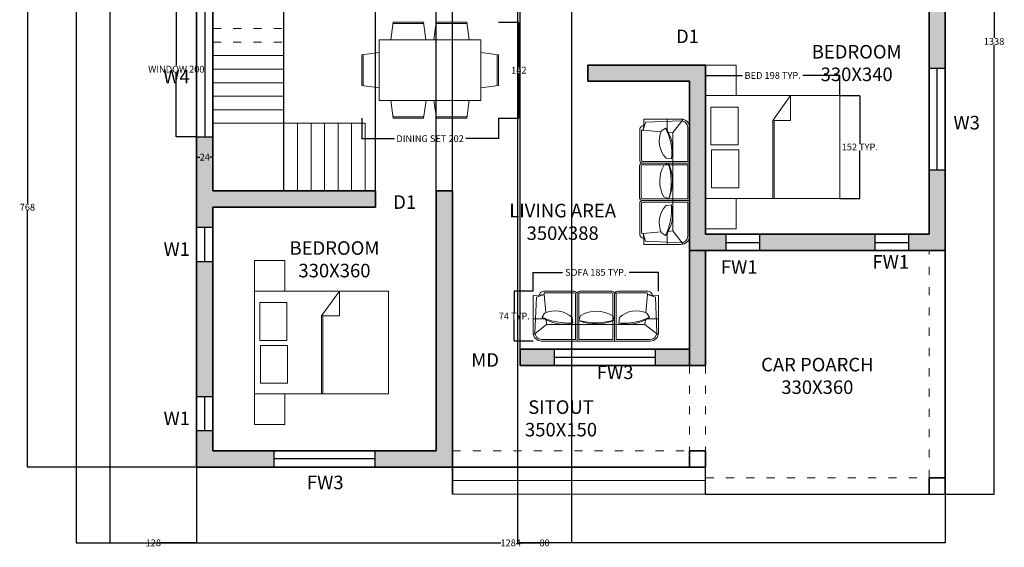
# Model space of a CAD drawing. Units: centimetres. Extents: x 1399 to 2860, y -110 to 1386.
# Tile 1 of 3: x 1399 to 2854, y -110 to 670. Entities that reach past the tile are written whole.
import ezdxf

# ---------------------------------------------------------------- set-up
doc = ezdxf.new("R2010")
doc.units = ezdxf.units.CM
doc.header["$MEASUREMENT"] = 0
doc.linetypes.add('ACAD_ISO03W100', pattern=[30, 12, -18])
for name, color, linetype, lineweight in [('A-ANNO-DIMS', 2, 'Continuous', 18), ('A-ANNO-TEXT', 7, 'Continuous', 18), ('A-AREA-IDEN', 7, 'Continuous', 25), ('A-COLS', 7, 'Continuous', 35), ('A-FLOR', 7, 'Continuous', 25), ('A-FLOR-OVHD', 8, 'ACAD_ISO03W100', 18), ('A-FLOR-STRS', 7, 'Continuous', 18), ('A-FLOR-STRS-OVHD', 8, 'ACAD_ISO03W100', 18), ('A-FURN', 8, 'Continuous', 18), ('A-GLAZ', 4, 'Continuous', 25), ('A-WALL', 7, 'Continuous', 35), ('A-WALL-PATT', 252, 'Continuous', 13)]:
    doc.layers.add(name, color=color, linetype=linetype, lineweight=lineweight)
doc.styles.get("Standard").update_dxf_attribs({"font": 'arial.ttf'})
doc.dimstyles.get("Standard").update_dxf_attribs({"dimtxt": 10, "dimasz": 0.18, "dimexe": 0.18, "dimexo": 0.0625, "dimgap": 0.09, "dimtad": 0, "dimtih": 1, "dimtoh": 1, "dimdec": 4, "dimzin": 0, "dimdsep": 46, "dimtxsty": 'Standard', "dimcen": 0.09, "dimadec": 0, "dimazin": 0, "dimtfac": 1, "dimtdec": 4, "dimtofl": 0, "dimtmove": 0, "dimatfit": 3, "dimfxl": 1, "dimtolj": 1, "dimtzin": 0, "dimarcsym": 0})

# ---------------------------------------------------------------- blocks, each defined once
blk = doc.blocks.new('v')
blk.add_line((1187.1, 1404.2), (1237.1, 1404.2))
blk.add_lwpolyline([(1187.1, 1392.2), (1237.1, 1392.2), (1237.1, 1416.2), (1187.1, 1416.2)], close=True)
blk = doc.blocks.new('w3')
blk.add_line((1235.3, 1319.4), (1085.3, 1319.4))
blk.add_lwpolyline([(1085.3, 1307.4), (1235.3, 1307.4), (1235.3, 1331.4), (1085.3, 1331.4)], close=True)
blk = doc.blocks.new('A$C7EC0217F')
for p, q in [((0.135, 0.808), (0.711, 0.808)), ((0.711, 0.808), (0.711, 0.046)), ((0.711, 0.807), (1.319, 0.807)), ((0.711, 0.045), (0.711, 0.807)), ((1.319, 0.807), (1.319, 0.045)), ((1.32, 0.808), (1.32, 0.046)), ((1.896, 0.808), (1.32, 0.808)), ((0, 0.069), (0, 0.673)), ((0.218, 0.538), (0.004, 0.706)), ((0.027, 0.673), (0.047, 0.095)), ((0.135, 0.781), (0.684, 0.781)), ((0.684, 0.045), (0.684, 0.781)), ((0.738, 0.78), (1.292, 0.78)), ((0.738, 0.045), (0.738, 0.78)), ((1.292, 0.78), (1.292, 0.045)), ((1.346, 0.781), (1.346, 0.045)), ((1.896, 0.781), (1.346, 0.781)), ((1.813, 0.538), (2.027, 0.706)), ((2.004, 0.673), (1.977, 0.095)), ((2.031, 0.069), (2.031, 0.673)), ((0.212, 0.464), (0.218, 0.538)), ((0.218, 0.538), (0.711, 0.538)), ((0.632, 0.428), (0.644, 0.516)), ((0.711, 0.612), (0.711, 0.612)), ((0.711, 0.537), (1.319, 0.537)), ((1.32, 0.612), (1.319, 0.612)), ((1.813, 0.538), (1.32, 0.538)), ((1.399, 0.428), (1.388, 0.516)), ((1.819, 0.464), (1.813, 0.538)), ((0, 0.448), (0.185, 0.448)), ((0.144, 0.42), (0.187, 0.355)), ((0.18, 0.055), (0.203, 0.347)), ((0.711, 0.432), (0.711, 0.432)), ((0.712, 0.47), (0.742, 0.399)), ((1.261, 0.391), (1.288, 0.475)), ((1.32, 0.432), (1.319, 0.432)), ((1.852, 0.055), (1.828, 0.347)), ((1.887, 0.42), (1.845, 0.355)), ((2.031, 0.448), (1.847, 0.448)), ((0.1, 0.066), (0, 0.069)), ((0.047, 0.095), (0.18, 0.055)), ((0.1, 0.066), (0.18, 0.055)), ((0.181, 0.028), (0.18, 0.055)), ((0.666, 0.028), (0.181, 0.028)), ((0.666, 0.001), (0.181, 0.001)), ((1.274, 0.027), (0.756, 0.027)), ((1.274, 0), (0.756, 0)), ((1.365, 0.028), (1.85, 0.028)), ((1.365, 0.001), (1.85, 0.001)), ((1.85, 0.028), (1.852, 0.055)), ((1.977, 0.095), (1.852, 0.055)), ((1.932, 0.066), (1.852, 0.055)), ((1.932, 0.066), (2.031, 0.069))]:
    blk.add_line(p, q)
for centre, radius, start, end in [((0.135, 0.673), 0.135, 90, 180), ((1.896, 0.673), 0.135, 0, 90), ((0.135, 0.673), 0.108, 90, 180), ((1.896, 0.673), 0.108, 0, 90), ((0.493, -0.046), 0.581, 74.928, 126.7929), ((0.559, -0.39), 0.91, 84.6406, 117.0804), ((1.02, -0.477), 0.989, 74.3176, 108.1894), ((1.006, -0.207), 0.738, 67.5209, 113.4724), ((1.381, -1.331), 1.892, 91.8503, 91.8916), ((1.381, -1.331), 1.87, 91.8726, 91.9144), ((1.539, -0.046), 0.581, 53.2071, 105.072), ((1.446, -0.529), 1.046, 65.0725, 93.2065), ((0.356, 0.715), 0.398, 244.7866, 313.8058), ((1.314, -1.331), 1.892, 108.5655, 108.5801), ((1.314, -1.331), 1.87, 108.7972, 108.812), ((1.008, 0.84), 0.515, 238.8934, 299.3642), ((1.675, 0.715), 0.398, 226.1942, 295.2134), ((1.381, -1.391), 1.6, 92.1888, 92.2376), ((0.173, 0.074), 0.0734, 186.4251, 276.5821), ((0.666, 0.046), 0.045, 270, 0), ((0.666, 0.046), 0.018, 270, 0), ((0.756, 0.045), 0.045, 180, 270), ((0.756, 0.045), 0.018, 180, 270), ((1.274, 0.045), 0.045, 270, 0), ((1.274, 0.045), 0.018, 270, 0), ((1.381, -1.391), 1.51, 92.3193, 92.3711), ((1.365, 0.046), 0.045, 180, 270), ((1.365, 0.046), 0.018, 180, 270), ((1.859, 0.074), 0.0734, 263.4179, 353.5749)]:
    blk.add_arc(centre, radius, start, end)
blk = doc.blocks.new('BED')
for p, q in [((1734.1, 2886.7), (1849.5, 2886.7)), ((1734.1, 2884.7), (1849.5, 2884.7)), ((1849.5, 2886.7), (1886.1, 2860.2)), ((1886.1, 2860.2), (1849.5, 2886.7)), ((1849.5, 2886.7), (1849.5, 2860.2)), ((1849.5, 2860.2), (1886.1, 2860.2))]:
    blk.add_line(p, q)
for points in [[(1734.1, 2787.7), (1886.1, 2787.7), (1886.1, 2985.7), (1734.1, 2985.7)], [(1750, 2936.8), (1805.9, 2936.8), (1805.9, 2977), (1750, 2977)], [(1813.2, 2937.8), (1869.1, 2937.8), (1869.1, 2977.9), (1813.2, 2977.9)]]:
    blk.add_lwpolyline(points, close=True)
blk = doc.blocks.new('DINING')
for p, q in [((1379.7, 3775.6), (1376.2, 3749.7)), ((1379.7, 3775.6), (1424.7, 3775.6)), ((1379.7, 3773.6), (1424.7, 3773.6)), ((1424.7, 3775.6), (1428.2, 3749.7)), ((1443.5, 3775.6), (1440, 3749.7)), ((1443.5, 3775.6), (1488.5, 3775.6)), ((1443.5, 3773.6), (1488.5, 3773.6)), ((1488.5, 3775.6), (1492, 3749.7)), ((1376.2, 3749.7), (1428.2, 3749.7)), ((1440, 3749.7), (1492, 3749.7)), ((1333.4, 3727.2), (1359.3, 3730.7)), ((1333.4, 3682.2), (1333.4, 3727.2)), ((1335.4, 3682.2), (1335.4, 3727.2)), ((1359.3, 3678.7), (1359.3, 3730.7)), ((1509.3, 3730.7), (1509.3, 3678.7)), ((1535.2, 3727.2), (1509.3, 3730.7)), ((1533.2, 3727.2), (1533.2, 3682.2)), ((1535.2, 3727.2), (1535.2, 3682.2)), ((1333.4, 3682.2), (1359.3, 3678.7)), ((1535.2, 3682.2), (1509.3, 3678.7)), ((1428.3, 3659.7), (1376.3, 3659.7)), ((1379.8, 3633.8), (1376.3, 3659.7)), ((1424.8, 3633.8), (1428.3, 3659.7)), ((1492.1, 3659.7), (1440.1, 3659.7)), ((1443.6, 3633.8), (1440.1, 3659.7)), ((1488.6, 3633.8), (1492.1, 3659.7)), ((1424.8, 3635.8), (1379.8, 3635.8)), ((1424.8, 3633.8), (1379.8, 3633.8)), ((1488.6, 3635.8), (1443.6, 3635.8)), ((1488.6, 3633.8), (1443.6, 3633.8))]:
    blk.add_line(p, q)
blk.add_lwpolyline([(1359.3, 3659.7), (1509.3, 3659.7), (1509.3, 3749.7), (1359.3, 3749.7)], close=True)
blk = doc.blocks.new('W4')
blk.add_line((1292.5, 2297.5), (1492.5, 2297.5))
blk.add_lwpolyline([(1292.5, 2285.5), (1492.5, 2285.5), (1492.5, 2309.5), (1292.5, 2309.5)], close=True)
blk = doc.blocks.new('NIGHTSTAND-450')
blk.add_lwpolyline([(0, 45), (0, 0), (45, 0), (45, 45)], close=True)
blk = doc.blocks.new('*D21')
at = {"layer": 'A-ANNO-DIMS', "color": 0, "lineweight": -2, "transparency": 16777216}
for p, q in [((1660.7, 697), (1630.6, 697)), ((1630.8, 696.8), (1630.8, 602.3)), ((1630.8, 497.2), (1630.8, 591.7)), ((1660.7, 497), (1630.6, 497))]:
    blk.add_line(p, q, dxfattribs=at)
at = {"layer": 'A-ANNO-DIMS', "color": 0, "transparency": 16777216}
for points in [[(1630.8, 696.8), (1630.8, 696.8), (1630.8, 697)], [(1630.8, 497.2), (1630.8, 497.2), (1630.8, 497)]]:
    blk.add_solid(points, dxfattribs=at)
at = {"layer": 'Defpoints', "color": 0, "transparency": 16777216}
for p in [(1660.8, 697), (1630.8, 497), (1660.8, 497)]:
    blk.add_point(p, dxfattribs=at)
at = {"layer": 'A-ANNO-DIMS', "color": 0, "transparency": 16777216, "insert": (1630.8, 597), "char_height": 10, "attachment_point": 5}
blk.add_mtext('\\A1;WINDOW 200', dxfattribs=at)
blk = doc.blocks.new('*D22')
at = {"layer": 'A-ANNO-DIMS', "color": 0, "lineweight": -2, "transparency": 16777216}
for p, q in [((1660.8, 496.9), (1660.8, 466.8)), ((1684.8, 496.9), (1684.8, 466.8)), ((1661, 467), (1665.5, 467)), ((1684.6, 467), (1680.1, 467))]:
    blk.add_line(p, q, dxfattribs=at)
at = {"layer": 'A-ANNO-DIMS', "color": 0, "transparency": 16777216}
for points in [[(1661, 467), (1661, 467), (1660.8, 467)], [(1684.6, 467), (1684.6, 467), (1684.8, 467)]]:
    blk.add_solid(points, dxfattribs=at)
at = {"layer": 'Defpoints', "color": 0, "transparency": 16777216}
for p in [(1660.8, 497), (1684.8, 497), (1684.8, 467)]:
    blk.add_point(p, dxfattribs=at)
at = {"layer": 'A-ANNO-DIMS', "color": 0, "transparency": 16777216, "insert": (1672.8, 467), "char_height": 10, "attachment_point": 5}
blk.add_mtext('\\A1;24', dxfattribs=at)
blk = doc.blocks.new('*D23')
at = {"layer": 'A-ANNO-DIMS', "color": 0, "lineweight": -2, "transparency": 16777216}
for p, q in [((2412.8, 558.1), (2412.8, 587.9)), ((2413, 587.7), (2467.4, 587.7)), ((2610.6, 587.7), (2556.2, 587.7)), ((2610.8, 558.1), (2610.8, 587.9))]:
    blk.add_line(p, q, dxfattribs=at)
at = {"layer": 'A-ANNO-DIMS', "color": 0, "transparency": 16777216}
for points in [[(2413, 587.7), (2413, 587.7), (2412.8, 587.7)], [(2610.6, 587.7), (2610.6, 587.7), (2610.8, 587.7)]]:
    blk.add_solid(points, dxfattribs=at)
at = {"layer": 'Defpoints', "color": 0, "transparency": 16777216}
for p in [(2412.8, 587.7), (2412.8, 558), (2610.8, 558)]:
    blk.add_point(p, dxfattribs=at)
at = {"layer": 'A-ANNO-DIMS', "color": 0, "transparency": 16777216, "insert": (2511.8, 587.7), "char_height": 10, "attachment_point": 5}
blk.add_mtext('\\A1;BED 198 TYP.', dxfattribs=at)
blk = doc.blocks.new('*D24')
at = {"layer": 'A-ANNO-DIMS', "color": 0, "lineweight": -2, "transparency": 16777216}
for p, q in [((2610.9, 558), (2640.7, 558)), ((2640.5, 557.8), (2640.5, 487.2)), ((2640.5, 406.2), (2640.5, 476.8)), ((2610.9, 406), (2640.7, 406))]:
    blk.add_line(p, q, dxfattribs=at)
at = {"layer": 'A-ANNO-DIMS', "color": 0, "transparency": 16777216}
for points in [[(2640.5, 557.8), (2640.5, 557.8), (2640.5, 558)], [(2640.5, 406.2), (2640.5, 406.2), (2640.5, 406)]]:
    blk.add_solid(points, dxfattribs=at)
at = {"layer": 'Defpoints', "color": 0, "transparency": 16777216}
for p in [(2610.8, 558), (2640.5, 558), (2610.8, 406)]:
    blk.add_point(p, dxfattribs=at)
at = {"layer": 'A-ANNO-DIMS', "color": 0, "transparency": 16777216, "insert": (2640.5, 482), "char_height": 10, "attachment_point": 5}
blk.add_mtext('\\A1;152 TYP.', dxfattribs=at)
blk = doc.blocks.new('*D29')
at = {"layer": 'A-ANNO-DIMS', "color": 0, "lineweight": -2, "transparency": 16777216}
for p, q in [((2157.9, 269), (2157.9, 296.9)), ((2158.1, 296.7), (2201.2, 296.7)), ((2342.9, 296.7), (2299.7, 296.7)), ((2343, 269), (2343, 296.9))]:
    blk.add_line(p, q, dxfattribs=at)
at = {"layer": 'A-ANNO-DIMS', "color": 0, "transparency": 16777216}
for points in [[(2158.1, 296.7), (2158.1, 296.7), (2157.9, 296.7)], [(2342.9, 296.7), (2342.9, 296.7), (2343, 296.7)]]:
    blk.add_solid(points, dxfattribs=at)
at = {"layer": 'Defpoints', "color": 0, "transparency": 16777216}
for p in [(2157.9, 296.7), (2157.9, 268.9), (2343, 268.9)]:
    blk.add_point(p, dxfattribs=at)
at = {"layer": 'A-ANNO-DIMS', "color": 0, "transparency": 16777216, "insert": (2250.5, 296.7), "char_height": 10, "attachment_point": 5}
blk.add_mtext('\\A1;SOFA 185 TYP.', dxfattribs=at)
blk = doc.blocks.new('*D30')
at = {"layer": 'A-ANNO-DIMS', "color": 0, "lineweight": -2, "transparency": 16777216}
for p, q in [((2157.8, 268.9), (2130, 268.9)), ((2130.1, 268.8), (2130.1, 237.2)), ((2130.1, 195.4), (2130.1, 227)), ((2157.8, 195.2), (2130, 195.2))]:
    blk.add_line(p, q, dxfattribs=at)
at = {"layer": 'A-ANNO-DIMS', "color": 0, "transparency": 16777216}
for points in [[(2130.1, 268.8), (2130.2, 268.8), (2130.1, 268.9)], [(2130.1, 195.4), (2130.2, 195.4), (2130.1, 195.2)]]:
    blk.add_solid(points, dxfattribs=at)
at = {"layer": 'Defpoints', "color": 0, "transparency": 16777216}
for p in [(2157.9, 268.9), (2130.1, 195.2), (2157.9, 195.2)]:
    blk.add_point(p, dxfattribs=at)
at = {"layer": 'A-ANNO-DIMS', "color": 0, "transparency": 16777216, "insert": (2130.1, 232.1), "char_height": 10, "attachment_point": 5}
blk.add_mtext('\\A1;74 TYP.', dxfattribs=at)
blk = doc.blocks.new('*D31')
at = {"layer": 'A-ANNO-DIMS', "color": 0, "lineweight": -2, "transparency": 16777216}
for p, q in [((1904.8, 524.5), (1904.8, 494.1)), ((2106.6, 524.5), (2106.6, 494.1)), ((1905, 494.3), (1952.9, 494.3)), ((2106.4, 494.3), (2058.4, 494.3))]:
    blk.add_line(p, q, dxfattribs=at)
at = {"layer": 'A-ANNO-DIMS', "color": 0, "transparency": 16777216}
for points in [[(1905, 494.3), (1905, 494.3), (1904.8, 494.3)], [(2106.4, 494.3), (2106.4, 494.3), (2106.6, 494.3)]]:
    blk.add_solid(points, dxfattribs=at)
at = {"layer": 'Defpoints', "color": 0, "transparency": 16777216}
for p in [(1904.8, 524.6), (2106.6, 524.6), (2106.6, 494.3)]:
    blk.add_point(p, dxfattribs=at)
at = {"layer": 'A-ANNO-DIMS', "color": 0, "transparency": 16777216, "insert": (2005.7, 494.3), "char_height": 10, "attachment_point": 5}
blk.add_mtext('\\A1;DINING SET 202', dxfattribs=at)
blk = doc.blocks.new('*D32')
at = {"layer": 'A-ANNO-DIMS', "color": 0, "lineweight": -2, "transparency": 16777216}
for p, q in [((2106.6, 666.4), (2137, 666.4)), ((2136.8, 666.2), (2136.8, 600.6)), ((2136.8, 524.8), (2136.8, 590.4)), ((2106.6, 524.6), (2137, 524.6))]:
    blk.add_line(p, q, dxfattribs=at)
at = {"layer": 'A-ANNO-DIMS', "color": 0, "transparency": 16777216}
for points in [[(2136.8, 666.2), (2136.9, 666.2), (2136.8, 666.4)], [(2136.8, 524.8), (2136.9, 524.8), (2136.8, 524.6)]]:
    blk.add_solid(points, dxfattribs=at)
at = {"layer": 'Defpoints', "color": 0, "transparency": 16777216}
for p in [(2106.6, 666.4), (2136.8, 666.4), (2106.6, 524.6)]:
    blk.add_point(p, dxfattribs=at)
at = {"layer": 'A-ANNO-DIMS', "color": 0, "transparency": 16777216, "insert": (2136.8, 595.5), "char_height": 10, "attachment_point": 5}
blk.add_mtext('\\A1;142', dxfattribs=at)
blk = doc.blocks.new('*D37')
at = {"layer": 'A-ANNO-DIMS', "color": 0, "lineweight": -2, "transparency": 16777216}
for p, q in [((1482.8, 800.9), (1482.8, -103.2)), ((2766.8, -31.1), (2766.8, -103.2)), ((1483, -103), (2110.3, -103)), ((2766.6, -103), (2139.3, -103))]:
    blk.add_line(p, q, dxfattribs=at)
at = {"layer": 'A-ANNO-DIMS', "color": 0, "transparency": 16777216}
for points in [[(1483, -103), (1483, -103.1), (1482.8, -103)], [(2766.6, -103), (2766.6, -103.1), (2766.8, -103)]]:
    blk.add_solid(points, dxfattribs=at)
at = {"layer": 'Defpoints', "color": 0, "transparency": 16777216}
for p in [(1482.8, 801), (2766.8, -31), (2766.8, -103)]:
    blk.add_point(p, dxfattribs=at)
at = {"layer": 'A-ANNO-DIMS', "color": 0, "transparency": 16777216, "insert": (2124.8, -103), "char_height": 10, "attachment_point": 5}
blk.add_mtext('\\A1;1284', dxfattribs=at)
blk = doc.blocks.new('*D38')
at = {"layer": 'A-ANNO-DIMS', "color": 0, "lineweight": -2, "transparency": 16777216}
for p, q in [((2766.9, 1307), (2839, 1307)), ((2838.9, 1306.8), (2838.9, 643.2)), ((2838.9, -30.8), (2838.9, 632.8)), ((2766.9, -31), (2839, -31))]:
    blk.add_line(p, q, dxfattribs=at)
at = {"layer": 'A-ANNO-DIMS', "color": 0, "transparency": 16777216}
for points in [[(2838.8, 1306.8), (2838.9, 1306.8), (2838.9, 1307)], [(2838.8, -30.8), (2838.9, -30.8), (2838.9, -31)]]:
    blk.add_solid(points, dxfattribs=at)
at = {"layer": 'Defpoints', "color": 0, "transparency": 16777216}
for p in [(2766.8, 1307), (2838.9, 1307), (2766.8, -31)]:
    blk.add_point(p, dxfattribs=at)
at = {"layer": 'A-ANNO-DIMS', "color": 0, "transparency": 16777216, "insert": (2838.9, 638), "char_height": 10, "attachment_point": 5}
blk.add_mtext('\\A1;1338', dxfattribs=at)
blk = doc.blocks.new('*D41')
at = {"layer": 'A-ANNO-DIMS', "color": 0, "lineweight": -2, "transparency": 16777216}
for p, q in [((1532.8, 776.9), (1532.8, -103.2)), ((1660.8, 776.9), (1660.8, -103.2)), ((1533, -103), (1586.1, -103)), ((1660.6, -103), (1607.5, -103))]:
    blk.add_line(p, q, dxfattribs=at)
at = {"layer": 'A-ANNO-DIMS', "color": 0, "transparency": 16777216}
for points in [[(1533, -103), (1533, -103.1), (1532.8, -103)], [(1660.6, -103), (1660.6, -103.1), (1660.8, -103)]]:
    blk.add_solid(points, dxfattribs=at)
at = {"layer": 'Defpoints', "color": 0, "transparency": 16777216}
for p in [(1532.8, 777), (1660.8, 777), (1660.8, -103)]:
    blk.add_point(p, dxfattribs=at)
at = {"layer": 'A-ANNO-DIMS', "color": 0, "transparency": 16777216, "insert": (1596.8, -103), "char_height": 10, "attachment_point": 5}
blk.add_mtext('\\A1;128', dxfattribs=at)
blk = doc.blocks.new('*D43')
at = {"layer": 'A-ANNO-DIMS', "color": 0, "lineweight": -2, "transparency": 16777216}
for p, q in [((1924.8, 417.1), (1924.8, 1379.2)), ((1925, 1379.1), (1962.6, 1379.1)), ((2014.6, 1379.1), (1977, 1379.1)), ((2014.8, 417.1), (2014.8, 1379.2))]:
    blk.add_line(p, q, dxfattribs=at)
at = {"layer": 'A-ANNO-DIMS', "color": 0, "transparency": 16777216}
for points in [[(1925, 1379.1), (1925, 1379), (1924.8, 1379.1)], [(2014.6, 1379.1), (2014.6, 1379), (2014.8, 1379.1)]]:
    blk.add_solid(points, dxfattribs=at)
at = {"layer": 'Defpoints', "color": 0, "transparency": 16777216}
for p in [(2014.8, 1379.1), (1924.8, 417), (2014.8, 417)]:
    blk.add_point(p, dxfattribs=at)
at = {"layer": 'A-ANNO-DIMS', "color": 0, "transparency": 16777216, "insert": (1969.8, 1379.1), "char_height": 10, "attachment_point": 5}
blk.add_mtext('\\A1;90', dxfattribs=at)
blk = doc.blocks.new('*D44')
at = {"layer": 'A-ANNO-DIMS', "color": 0, "lineweight": -2, "transparency": 16777216}
for p, q in [((2134.8, 906.9), (2134.8, -103.2)), ((2214.8, 906.9), (2214.8, -103.2)), ((2135, -103), (2167.6, -103)), ((2214.6, -103), (2182, -103))]:
    blk.add_line(p, q, dxfattribs=at)
at = {"layer": 'A-ANNO-DIMS', "color": 0, "transparency": 16777216}
for points in [[(2135, -103), (2135, -103.1), (2134.8, -103)], [(2214.6, -103), (2214.6, -103.1), (2214.8, -103)]]:
    blk.add_solid(points, dxfattribs=at)
at = {"layer": 'Defpoints', "color": 0, "transparency": 16777216}
for p in [(2134.8, 907), (2214.8, 907), (2214.8, -103)]:
    blk.add_point(p, dxfattribs=at)
at = {"layer": 'A-ANNO-DIMS', "color": 0, "transparency": 16777216, "insert": (2174.8, -103), "char_height": 10, "attachment_point": 5}
blk.add_mtext('\\A1;80', dxfattribs=at)
blk = doc.blocks.new('*D45')
at = {"layer": 'A-ANNO-DIMS', "color": 0, "lineweight": -2, "transparency": 16777216}
for p, q in [((2038.8, 33.1), (2038.8, 1379.2)), ((2039, 1379.1), (2078.2, 1379.1)), ((2138.6, 1379.1), (2099.5, 1379.1)), ((2138.8, 183.1), (2138.8, 1379.2))]:
    blk.add_line(p, q, dxfattribs=at)
at = {"layer": 'A-ANNO-DIMS', "color": 0, "transparency": 16777216}
for points in [[(2039, 1379.1), (2039, 1379), (2038.8, 1379.1)], [(2138.6, 1379.1), (2138.6, 1379), (2138.8, 1379.1)]]:
    blk.add_solid(points, dxfattribs=at)
at = {"layer": 'Defpoints', "color": 0, "transparency": 16777216}
for p in [(2038.8, 1379.1), (2138.8, 183), (2038.8, 33)]:
    blk.add_point(p, dxfattribs=at)
at = {"layer": 'A-ANNO-DIMS', "color": 0, "transparency": 16777216, "insert": (2088.8, 1379.1), "char_height": 10, "attachment_point": 5}
blk.add_mtext('\\A1;100', dxfattribs=at)
blk = doc.blocks.new('*D48')
at = {"layer": 'A-ANNO-DIMS', "color": 0, "lineweight": -2, "transparency": 16777216}
for p, q in [((1684.8, 417.1), (1684.8, 1379.2)), ((1685, 1379.1), (1726.6, 1379.1)), ((1789.6, 1379.1), (1748, 1379.1)), ((1789.8, 417.1), (1789.8, 1379.2))]:
    blk.add_line(p, q, dxfattribs=at)
at = {"layer": 'A-ANNO-DIMS', "color": 0, "transparency": 16777216}
for points in [[(1685, 1379.1), (1685, 1379), (1684.8, 1379.1)], [(1789.6, 1379.1), (1789.6, 1379), (1789.8, 1379.1)]]:
    blk.add_solid(points, dxfattribs=at)
at = {"layer": 'Defpoints', "color": 0, "transparency": 16777216}
for p in [(1789.8, 1379.1), (1684.8, 417), (1789.8, 417)]:
    blk.add_point(p, dxfattribs=at)
at = {"layer": 'A-ANNO-DIMS', "color": 0, "transparency": 16777216, "insert": (1737.3, 1379.1), "char_height": 10, "attachment_point": 5}
blk.add_mtext('\\A1;105', dxfattribs=at)
blk = doc.blocks.new('*D50')
at = {"layer": 'A-ANNO-DIMS', "color": 0, "lineweight": -2, "transparency": 16777216}
for p, q in [((1660.7, 777), (1410.6, 777)), ((1410.8, 776.8), (1410.8, 398.2)), ((1410.8, 9.2), (1410.8, 387.8)), ((1660.7, 9), (1410.6, 9))]:
    blk.add_line(p, q, dxfattribs=at)
at = {"layer": 'A-ANNO-DIMS', "color": 0, "transparency": 16777216}
for points in [[(1410.7, 776.8), (1410.8, 776.8), (1410.8, 777)], [(1410.7, 9.2), (1410.8, 9.2), (1410.8, 9)]]:
    blk.add_solid(points, dxfattribs=at)
at = {"layer": 'Defpoints', "color": 0, "transparency": 16777216}
for p in [(1410.8, 777), (1660.8, 777), (1660.8, 9)]:
    blk.add_point(p, dxfattribs=at)
at = {"layer": 'A-ANNO-DIMS', "color": 0, "transparency": 16777216, "insert": (1410.8, 393), "char_height": 10, "attachment_point": 5}
blk.add_mtext('\\A1;768', dxfattribs=at)

msp = doc.modelspace()

# ---------------------------------------------------------------- hatches: boundary and pattern name
at = {"layer": 'A-WALL-PATT'}
h = msp.add_hatch(color=256, dxfattribs=at)
h.dxf.hatch_style = 1
h.paths.add_polyline_path([(1581.8022, 1155.0098), (1532.8022, 1155.0098), (1532.8022, 1081.0098), (1556.8022, 1081.0098), (1556.8022, 1131.0098), (1581.8022, 1131.0098)])
h.paths.add_polyline_path([(1556.8022, 931.0098), (1532.8022, 931.0098), (1532.8022, 881.0098), (1556.8022, 881.0098)])
h.paths.add_polyline_path([(1820.8022, 1155.0098), (1681.8022, 1155.0098), (1681.8022, 1131.0098), (1706.8022, 1131.0098), (1706.8022, 881.0098), (1730.8022, 881.0098), (1730.8022, 1131.0098), (1820.8022, 1131.0098)])
h.paths.add_polyline_path([(2119.8022, 1155.0098), (1970.8022, 1155.0098), (1970.8022, 1131.0098), (2060.8022, 1131.0098), (2060.8022, 777.0098), (2084.8022, 777.0098), (2084.8022, 907.0098), (2134.8022, 907.0098), (2134.8022, 931.0098), (2084.8022, 931.0098), (2084.8022, 1131.0098), (2119.8022, 1131.0098)])
h.paths.add_polyline_path([(2283.8022, 1155.0098), (2179.8022, 1155.0098), (2179.8022, 1131.0098), (2214.8022, 1131.0098), (2214.8022, 907.0098), (2388.8022, 907.0098), (2388.8022, 857.0098), (2412.8022, 857.0098), (2412.8022, 931.0098), (2238.8022, 931.0098), (2238.8022, 1131.0098), (2283.8022, 1131.0098)])
h.paths.add_polyline_path([(2388.8022, 1155.0098), (2343.8022, 1155.0098), (2343.8022, 1131.0098), (2388.8022, 1131.0098)], flags=17)
h.paths.add_polyline_path([(2412.8022, 1283.0098), (2442.8022, 1283.0098), (2442.8022, 1307.0098), (2388.8022, 1307.0098), (2388.8022, 1011.0098), (2412.8022, 1011.0098)])
h.paths.add_polyline_path([(2662.8022, 1307.0098), (2492.8022, 1307.0098), (2492.8022, 1283.0098), (2662.8022, 1283.0098)])
h.paths.add_polyline_path([(2766.8022, 1307.0098), (2712.8022, 1307.0098), (2712.8022, 1283.0098), (2742.8022, 1283.0098), (2742.8022, 1157.0098), (2766.8022, 1157.0098)])
h.paths.add_polyline_path([(2766.8022, 1007.0098), (2742.8022, 1007.0098), (2742.8022, 881.0098), (2502.8022, 881.0098), (2502.8022, 717.0098), (2388.8022, 717.0098), (2388.8022, 693.0098), (2526.8022, 693.0098), (2526.8022, 857.0098), (2742.8022, 857.0098), (2742.8022, 817.0098), (2766.8022, 817.0098)])
h.paths.add_polyline_path([(2766.8022, 757.0098), (2742.8022, 757.0098), (2742.8022, 717.0098), (2606.8022, 717.0098), (2606.8022, 693.0098), (2742.8022, 693.0098), (2742.8022, 598.0098), (2766.8022, 598.0098)])
h.paths.add_polyline_path([(2442.8022, 353.0098), (2412.8022, 353.0098), (2412.8022, 603.0098), (2238.8022, 603.0098), (2238.8022, 579.0098), (2388.8022, 579.0098), (2388.8022, 512.2445, -0.029168985), (2388.8858, 510.8126), (2388.8858, 458.2748), (2388.8022, 458.2748), (2388.8022, 402.9002), (2388.8024, 402.776), (2388.8858, 402.776), (2388.8858, 350.2798, -0.029168985), (2388.8022, 348.8479), (2388.8022, 329.0098), (2442.8022, 329.0098)])
h.paths.add_polyline_path([(2662.8022, 353.0098), (2492.8022, 353.0098), (2492.8022, 329.0098), (2662.8022, 329.0098)])
h.paths.add_polyline_path([(2412.8022, 329.0098), (2388.8022, 329.0098), (2388.8022, 159.0098), (2412.8022, 159.0098)])
h.paths.add_polyline_path([(2388.8022, 183.0098), (2338.8022, 183.0098), (2338.8022, 159.0098), (2388.8022, 159.0098)])
h.paths.add_polyline_path([(2188.8022, 183.0098), (2138.8022, 183.0098), (2138.8022, 159.0098), (2188.8022, 159.0098)])
h.paths.add_polyline_path([(2038.8022, 417.0098), (2014.8022, 417.0098), (2014.8022, 33.0098), (1924.8022, 33.0098), (1924.8022, 9.0098), (2038.8022, 9.0098)])
h.paths.add_polyline_path([(1774.8022, 33.0098), (1684.8022, 33.0098), (1684.8022, 63.0098), (1660.8022, 63.0098), (1660.8022, 9.0098), (1774.8022, 9.0098)])
h.paths.add_polyline_path([(1684.8022, 313.0098), (1660.8022, 313.0098), (1660.8022, 113.0098), (1684.8022, 113.0098)])
h.paths.add_polyline_path([(1924.8022, 417.0098), (1684.8022, 417.0098), (1684.8022, 497.0098), (1660.8022, 497.0098), (1660.8022, 363.0098), (1684.8022, 363.0098), (1684.8022, 393.0098), (1924.8022, 393.0098)])
h.paths.add_polyline_path([(1684.8022, 777.0098), (1660.8022, 777.0098), (1660.8022, 697.0098), (1684.8022, 697.0098)])
h.paths.add_polyline_path([(1970.8022, 801.0098), (1532.8022, 801.0098), (1532.8022, 777.0098), (1970.8022, 777.0098)])
h = msp.add_hatch(color=256, dxfattribs=at)
h.dxf.hatch_style = 1
h.paths.add_polyline_path([(2766.8022, 448.0098), (2742.8022, 448.0098), (2742.8022, 353.0098), (2712.8022, 353.0098), (2712.8022, 329.0098), (2766.8022, 329.0098)])

# ---------------------------------------------------------------- linework, layer by layer
at = {"layer": 'A-COLS'}
for p, q in [((2388.8022, 9.0098), (2388.8022, 33.0098)), ((2388.8022, 33.0098), (2412.8022, 33.0098)), ((2412.8022, 33.0098), (2412.8022, 9.0098)), ((2742.8022, -6.9902), (2766.8022, -6.9902)), ((2742.8022, -6.9902), (2742.8022, -30.9902))]:
    msp.add_line(p, q, dxfattribs=at)
at = {"layer": 'A-FLOR'}
for q in [(2412.8022, 9.0098), (2766.8022, -30.9902)]:
    msp.add_line((2412.8022, -30.9902), q, dxfattribs=at)
at = {"layer": 'A-FLOR-OVHD'}
for p, q in [((2742.8022, -6.9902), (2742.8022, 329.0098)), ((2388.8022, 159.0098), (2388.8022, 33.0098)), ((2412.8022, 159.0098), (2412.8022, 33.0098)), ((2038.8022, 33.0098), (2388.8022, 33.0098)), ((2412.8022, -6.9902), (2742.8022, -6.9902))]:
    msp.add_line(p, q, dxfattribs=at)
at = {"layer": 'A-FLOR-STRS'}
for p, q in [((1789.8022, 417.0098), (1789.8022, 677.0098)), ((1684.8022, 617.0098), (1789.8022, 617.0098)), ((1684.8022, 597.0098), (1789.8022, 597.0098)), ((1684.8022, 577.0098), (1789.8022, 577.0098)), ((1684.8022, 557.0098), (1789.8022, 557.0098)), ((1684.8022, 537.0098), (1789.8022, 537.0098)), ((1684.8022, 517.0098), (1909.8022, 517.0098)), ((1809.8022, 417.0098), (1809.8022, 517.0098)), ((1829.8022, 417.0098), (1829.8022, 517.0098)), ((1849.8022, 417.0098), (1849.8022, 517.0098)), ((1869.8022, 417.0098), (1869.8022, 517.0098)), ((1889.8022, 417.0098), (1889.8022, 517.0098)), ((1909.8022, 417.0098), (1909.8022, 517.0098)), ((2038.8022, -10.9902), (2412.8022, -10.9902)), ((2038.8022, -30.9902), (2412.8022, -30.9902))]:
    msp.add_line(p, q, dxfattribs=at)
at = {"layer": 'A-FLOR-STRS-OVHD'}
for p, q in [((1684.8022, 657.0098), (1789.8022, 657.0098)), ((1684.8022, 637.0098), (1789.8022, 637.0098))]:
    msp.add_line(p, q, dxfattribs=at)
at = {"layer": 'A-WALL'}
for p, q in [((2766.8022, -30.9902), (2766.8022, 1307.0098)), ((1660.8022, 9.0098), (1660.8022, 777.0098)), ((1684.8022, 417.0098), (1684.8022, 777.0098)), ((2742.8022, 353.0098), (2742.8022, 693.0098)), ((2238.8022, 603.0098), (2412.8022, 603.0098)), ((2238.8022, 579.0098), (2238.8022, 603.0098)), ((2412.8022, 353.0098), (2412.8022, 603.0098)), ((2238.8022, 579.0098), (2388.8022, 579.0098)), ((2388.8022, 159.0098), (2388.8022, 579.0098)), ((1684.8022, 417.0098), (1924.8022, 417.0098)), ((1924.8022, 393.0098), (1924.8022, 417.0098)), ((2014.8022, 33.0098), (2014.8022, 417.0098)), ((2014.8022, 417.0098), (2038.8022, 417.0098)), ((2038.8022, -30.9902), (2038.8022, 417.0098)), ((1684.8022, 33.0098), (1684.8022, 393.0098)), ((1684.8022, 393.0098), (1924.8022, 393.0098)), ((2412.8022, 353.0098), (2742.8022, 353.0098)), ((2388.8022, 329.0098), (2766.8022, 329.0098)), ((2412.8022, 159.0098), (2412.8022, 329.0098)), ((2138.8022, 183.0098), (2388.8022, 183.0098)), ((2138.8022, 159.0098), (2138.8022, 183.0098)), ((2138.8022, 159.0098), (2412.8022, 159.0098)), ((1684.8022, 33.0098), (2014.8022, 33.0098)), ((1660.8022, 9.0098), (2412.8022, 9.0098))]:
    msp.add_line(p, q, dxfattribs=at)

# ---------------------------------------------------------------- block references
at = {"layer": 'A-FURN'}
for name, p in [('DINING', (571.3542, -3109.2497)), ('NIGHTSTAND-450', (2412.8022, 558.0098)), ('NIGHTSTAND-450', (2412.8022, 361.0098)), ('NIGHTSTAND-450', (1746.2698, 269.0098)), ('NIGHTSTAND-450', (1746.2698, 72.0098))]:
    msp.add_blockref(name, p, dxfattribs=at)
at = {"layer": 'A-FURN', "rotation": 89.99999999999999}
for p in [(5398.5411, -1328.1299), (4732.0087, -1617.1299)]:
    msp.add_blockref('BED', p, dxfattribs=at)
at = {"layer": 'A-FURN', "xscale": 91.13924050632912, "yscale": 91.13924050632912, "zscale": 91.13924050632912}
for p, rotation in [((2315.2902, 523.1164), 270), ((2343.0437, 268.8256), 180)]:
    msp.add_blockref('A$C7EC0217F', p, dxfattribs=dict(at, rotation=rotation))
at = {"layer": 'A-GLAZ'}
for name, p, rotation in [('W4', (-624.7289, 1989.489), 270), ('w3', (1435.392, 1683.3567), 270), ('v', (3076.9917, -874.1204), 90), ('v', (3076.9917, -1124.1204), 90)]:
    msp.add_blockref(name, p, dxfattribs=dict(at, rotation=rotation))
for name, p in [('v', (1255.672, -1063.1797)), ('v', (1475.672, -1063.1797)), ('w3', (1103.4552, -1148.4003)), ('w3', (689.4552, -1298.4003))]:
    msp.add_blockref(name, p, dxfattribs=at)

# ---------------------------------------------------------------- texts
at = {"layer": 'A-ANNO-TEXT', "char_height": 20, "attachment_point": 1}
for s, width, insert in [('D1', 103.726959, (2369.0492, 655.5489)), ('W4', 163.588182, (1611.55, 596.0898)), ('W3', 163.588182, (2778.8214, 527.9324)), ('D1', 103.726959, (1951.2323, 410.5829)), ('W1', 163.588182, (1611.9018, 341.0735)), ('FW1', 163.588182, (2659.1646, 322.2548)), ('FW1', 163.588182, (2435.2646, 314.576)), ('MD', 103.726959, (2066.5579, 177.2869)), ('FW3', 163.588182, (2252.0031, 159.0098)), ('W1', 163.588182, (1611.9018, 90.986)), ('FW3', 163.588182, (1823.7392, -3.7296))]:
    msp.add_mtext_dynamic_manual_height_columns(s, width=width, gutter_width=1, heights=[0], dxfattribs=dict(at, insert=insert))
at = {"layer": 'A-AREA-IDEN', "char_height": 20, "attachment_point": 1}
for s, heights, insert in [('\\pxqc;BEDROOM\\P330X340', [0], (2402.564, 632.6851)), ('\\pxqc;LIVING AREA\\P350X388', [0], (1968.187, 397.9884)), ('\\pxqc;BEDROOM\\P330X360', [0], (1631.0837, 342.6671)), ('\\pxqc;CAR POARCH\\P330X360', [64.477], (2344.4804, 170.4055)), ('\\pxqc;SITOUT\\P350X150', [64.477], (1965.8127, 107.6068))]:
    msp.add_mtext_dynamic_manual_height_columns(s, width=466.660539, gutter_width=1, heights=heights, dxfattribs=dict(at, insert=insert))

# ---------------------------------------------------------------- dimensions: what is measured, and where the dimension line sits
at = {"layer": 'A-ANNO-DIMS'}
for base, p1, p2, picture, middle in [((1789.8022, 1379.0598), (1684.8022, 417.0098), (1789.8022, 417.0098), '*D48', (1737.3022, 1379.0598)), ((2014.8022, 1379.0598), (1924.8022, 417.0098), (2014.8022, 417.0098), '*D43', (1969.8022, 1379.0598)), ((2038.8022, 1379.0598), (2138.8022, 183.0098), (2038.8022, 33.0098), '*D45', (2088.8022, 1379.0598)), ((2214.8022, -103.0402), (2134.8022, 907.0098), (2214.8022, 907.0098), '*D44', (2174.8022, -103.0402)), ((2766.8022, -103.0402), (1482.8022, 801.0098), (2766.8022, -30.9902), '*D37', (2124.8022, -103.0402)), ((1660.8022, -103.0402), (1532.8022, 777.0098), (1660.8022, 777.0098), '*D41', (1596.8022, -103.0402)), ((1684.8022, 467.0098), (1660.8022, 497.0098), (1684.8022, 497.0098), '*D22', (1672.8022, 467.0098))]:
    dim = msp.add_linear_dim(base=base, p1=p1, p2=p2, dimstyle='Standard', override={"dimdec": 0, "dimlfac": 1, "dimrnd": 0, "dimzin": 0, "dimdsep": 46, "dimlunit": 2}, dxfattribs=at)
    dim.commit()
    dim.dimension.update_dxf_attribs({"geometry": picture, "text_midpoint": middle})
for base, p1, p2, picture, middle in [((2838.8522, 1307.0098), (2766.8022, -30.9902), (2766.8022, 1307.0098), '*D38', (2838.8522, 638.0098)), ((1410.7522, 777.0098), (1660.8022, 9.0098), (1660.8022, 777.0098), '*D50', (1410.7522, 393.0098)), ((2136.8439, 666.3658), (2106.5748, 524.5719), (2106.5748, 666.3658), '*D32', (2136.8439, 595.4688))]:
    dim = msp.add_linear_dim(base=base, p1=p1, p2=p2, angle=90, dimstyle='Standard', override={"dimdec": 0, "dimlfac": 1, "dimrnd": 0, "dimzin": 0, "dimdsep": 46, "dimlunit": 2}, dxfattribs=at)
    dim.commit()
    dim.dimension.update_dxf_attribs({"geometry": picture, "text_midpoint": middle})
for base, p1, p2, angle, text, picture, middle in [((1630.8022, 497.0098), (1660.8022, 697.0098), (1660.8022, 497.0098), 270, 'WINDOW <>', '*D21', (1630.8022, 597.0098)), ((2412.8022, 587.7098), (2610.8022, 558.0098), (2412.8022, 558.0098), 180, 'BED <> TYP.', '*D23', (2511.8022, 587.7098)), ((2640.5022, 558.0098), (2610.8022, 406.0098), (2610.8022, 558.0098), 90, '<> TYP.', '*D24', (2640.5022, 482.0098)), ((2157.9033, 296.7168), (2343.0437, 268.9458), (2157.9033, 268.9458), 180, 'SOFA <> TYP.', '*D29', (2250.4735, 296.7168)), ((2130.1322, 195.23), (2157.9033, 268.9458), (2157.9033, 195.23), 270, '<> TYP.', '*D30', (2130.1322, 232.0879))]:
    dim = msp.add_linear_dim(base=base, p1=p1, p2=p2, angle=angle, text=text, dimstyle='Standard', override={"dimdec": 0, "dimlfac": 1, "dimrnd": 0, "dimzin": 0, "dimdsep": 46, "dimlunit": 2}, dxfattribs=at)
    dim.commit()
    dim.dimension.update_dxf_attribs({"geometry": picture, "text_midpoint": middle})
dim = msp.add_linear_dim(base=(2106.5748, 494.3028), p1=(1904.781, 524.5719), p2=(2106.5748, 524.5719), text='DINING SET <>', dimstyle='Standard', override={"dimdec": 0, "dimlfac": 1, "dimrnd": 0, "dimzin": 0, "dimdsep": 46, "dimlunit": 2}, dxfattribs=at)
dim.commit()
dim.dimension.update_dxf_attribs({"geometry": '*D31', "text_midpoint": (2005.6779, 494.3028)})

doc.saveas('drawing.dxf')
